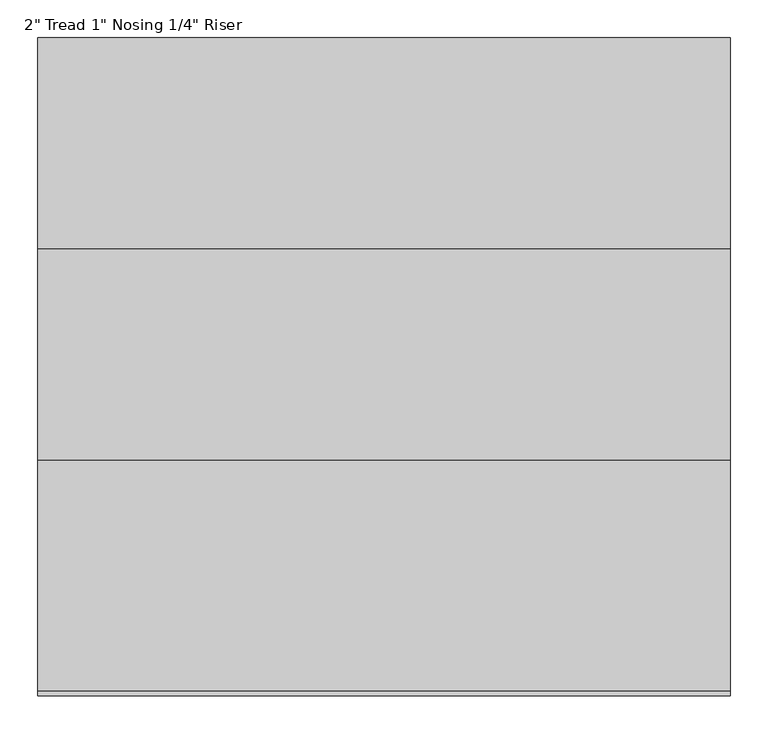
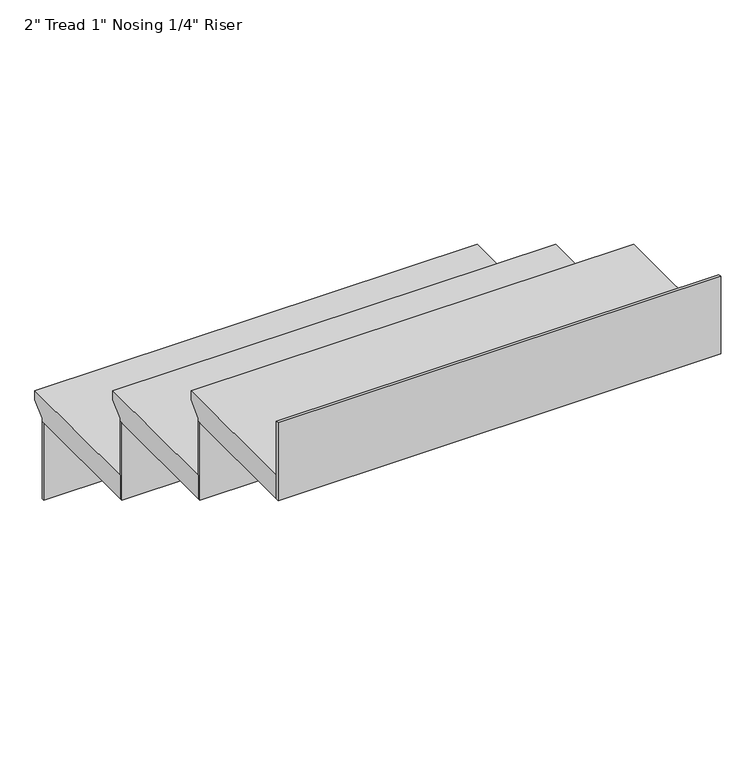
"""IFC4 building model written with IfcOpenShell, lengths in millimetres: stair flight geometry."""

from ifc_helpers import new_model, si_unit, frame, origin, place, context, project, spatial, polyline, outline, extrude, source, transform, mapped, element, save


def stair_flight_5a0a31fc(model_context):
    return source(origin(), model_context, "Body", "SweptSolid", [
        extrude(outline(polyline([(-19826.9851539, 33870.6172466), (-19522.1851539, 33870.6172466), (-19522.1851539, 33851.5672466), (-19547.5851539, 33826.1672466), (-19547.5851539, 33819.8172466), (-19826.9851539, 33819.8172466), (-19826.9851539, 33870.6172466)])), frame((-2296.6415084, 0.0, 0.0), z_axis=(1.0, 0.0, 0.0), x_axis=(0.0, 1.0, 0.0)), (0.0, 0.0, 1.0), 914.4),
        extrude(outline(polyline([(-2296.6415084, -19553.9351539), (-2296.6415084, -19547.5851539), (-1382.2415084, -19547.5851539), (-1382.2415084, -19553.9351539), (-2296.6415084, -19553.9351539)])), frame((0.0, 0.0, 33650.4839133), z_axis=(0.0, 0.0, 1.0), x_axis=(1.0, 0.0, 0.0)), (0.0, 0.0, 1.0), 169.3333333),
        extrude(outline(polyline([(-2296.6415084, -19833.3351539), (-2296.6415084, -19826.9851539), (-1382.2415084, -19826.9851539), (-1382.2415084, -19833.3351539), (-2296.6415084, -19833.3351539)])), frame((0.0, 0.0, 33819.8172466), z_axis=(0.0, 0.0, 1.0), x_axis=(1.0, 0.0, 0.0)), (0.0, 0.0, 1.0), 169.3333333),
        extrude(outline(polyline([(-20106.3851539, 34039.9505799), (-19801.5851539, 34039.9505799), (-19801.5851539, 34020.9005799), (-19826.9851539, 33995.5005799), (-19826.9851539, 33989.1505799), (-20106.3851539, 33989.1505799), (-20106.3851539, 34039.9505799)])), frame((-2296.6415084, 0.0, 0.0), z_axis=(1.0, 0.0, 0.0), x_axis=(0.0, 1.0, 0.0)), (0.0, 0.0, 1.0), 914.4),
        extrude(outline(polyline([(-2296.6415084, -20112.7351539), (-2296.6415084, -20106.3851539), (-1382.2415084, -20106.3851539), (-1382.2415084, -20112.7351539), (-2296.6415084, -20112.7351539)])), frame((0.0, 0.0, 33989.1505799), z_axis=(0.0, 0.0, 1.0), x_axis=(1.0, 0.0, 0.0)), (0.0, 0.0, 1.0), 169.3333333),
        extrude(outline(polyline([(-2296.6415084, -20392.1351539), (-2296.6415084, -20385.7851539), (-1382.2415084, -20385.7851539), (-1382.2415084, -20392.1351539), (-2296.6415084, -20392.1351539)])), frame((0.0, 0.0, 34158.4839133), z_axis=(0.0, 0.0, 1.0), x_axis=(1.0, 0.0, 0.0)), (0.0, 0.0, 1.0), 169.3333333),
        extrude(outline(polyline([(-20385.7851539, 34209.2839133), (-20080.9851539, 34209.2839133), (-20080.9851539, 34190.2339133), (-20106.3851539, 34164.8339133), (-20106.3851539, 34158.4839133), (-20385.7851539, 34158.4839133), (-20385.7851539, 34209.2839133)])), frame((-2296.6415084, 0.0, 0.0), z_axis=(1.0, 0.0, 0.0), x_axis=(0.0, 1.0, 0.0)), (0.0, 0.0, 1.0), 914.4),
    ])


if __name__ == "__main__":
    model = new_model("IFC4")
    model_context = context("Model", 3, world=origin())
    ifc_project = project(units=[si_unit("LENGTHUNIT", "METRE", prefix="MILLI")], contexts=[model_context])
    site = spatial("IfcSite", under=ifc_project)
    building = spatial("IfcBuilding", under=site)
    placement = place(None, origin())
    stair_flight_shape = stair_flight_5a0a31fc(model_context)
    element("IfcStairFlight", 1, ObjectType="2\" Tread 1\" Nosing 1/4\" Riser", at=placement, inside=building, context=model_context, shape_type="MappedRepresentation", body=[
        mapped(stair_flight_shape, transform((0.0, 0.0, 0.0), x_axis=(1.0, 0.0, 0.0), y_axis=(0.0, 1.0, 0.0), z_axis=(0.0, 0.0, 1.0))),
    ])
    save(model, "model.ifc")
